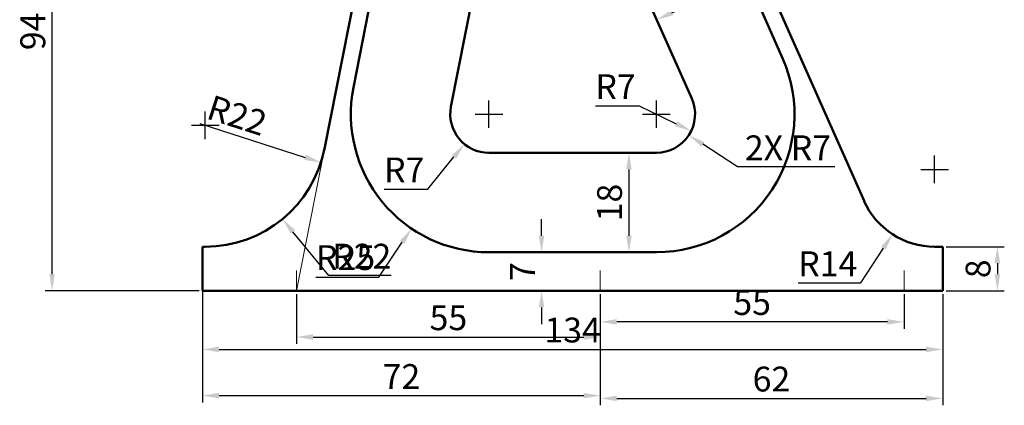
# Model space of a CAD drawing. Units: millimetres. Extents: x 43 to 233, y 2 to 211.
# Tile 1 of 2: x 43 to 221, y 2 to 72. Entities that reach past the tile are written whole.
import ezdxf

# ---------------------------------------------------------------- set-up
doc = ezdxf.new("R2010")
doc.units = ezdxf.units.MM
for name, color, linetype, lineweight in [('M-CONS', 8, 'Continuous', 13), ('M-DIMS', 2, 'Continuous', 25), ('M-OUTL', 7, 'Continuous', 50)]:
    doc.layers.add(name, color=color, linetype=linetype, lineweight=lineweight)
doc.styles.get("Standard").update_dxf_attribs({"font": 'arial.ttf'})
doc.dimstyles.new('ISO-25', dxfattribs={"dimtxt": 4.5, "dimasz": 3, "dimexe": 1.25, "dimexo": 0.625, "dimtad": 1, "dimtoh": 1, "dimdec": 0, "dimtxsty": 'Standard', "dimcen": 2.5, "dimadec": 0, "dimazin": 0, "dimtfac": 1, "dimtdec": 0, "dimtofl": 0, "dimtmove": 0, "dimatfit": 3, "dimfxl": 1, "dimarcsym": 0})

# ---------------------------------------------------------------- blocks, each defined once
blk = doc.blocks.new('*D1')
at = {"layer": 'Defpoints', "color": 0, "transparency": 16777216}
for p in [(75.97, 24.51), (147.97, 23.16), (147.97, 4.19)]:
    blk.add_point(p, dxfattribs=at)
at = {"layer": 'M-DIMS', "color": 0, "lineweight": -2, "transparency": 16777216}
for p, q in [((75.97, 23.88), (75.97, 2.94)), ((147.97, 22.54), (147.97, 2.94)), ((78.97, 4.19), (144.97, 4.19))]:
    blk.add_line(p, q, dxfattribs=at)
at = {"layer": 'M-DIMS', "color": 0, "transparency": 16777216}
for points in [[(78.97, 4.69), (78.97, 3.69), (75.97, 4.19)], [(144.97, 4.69), (144.97, 3.69), (147.97, 4.19)]]:
    blk.add_solid(points, dxfattribs=at)
at = {"layer": 'M-DIMS', "color": 0, "transparency": 16777216, "insert": (111.97, 7.07), "char_height": 4.5, "attachment_point": 5}
blk.add_mtext('72', dxfattribs=at)
blk = doc.blocks.new('*D2')
at = {"layer": 'Defpoints', "color": 0, "transparency": 16777216}
for p in [(147.97, 23.16), (209.97, 23.16), (209.97, 3.69)]:
    blk.add_point(p, dxfattribs=at)
at = {"layer": 'M-DIMS', "color": 0, "lineweight": -2, "transparency": 16777216}
for p, q in [((147.97, 22.54), (147.97, 2.44)), ((209.97, 22.54), (209.97, 2.44)), ((150.97, 3.69), (206.97, 3.69))]:
    blk.add_line(p, q, dxfattribs=at)
at = {"layer": 'M-DIMS', "color": 0, "transparency": 16777216}
for points in [[(150.97, 4.19), (150.97, 3.19), (147.97, 3.69)], [(206.97, 4.19), (206.97, 3.19), (209.97, 3.69)]]:
    blk.add_solid(points, dxfattribs=at)
at = {"layer": 'M-DIMS', "color": 0, "transparency": 16777216, "insert": (178.97, 6.61), "char_height": 4.5, "attachment_point": 5}
blk.add_mtext('62', dxfattribs=at)
blk = doc.blocks.new('*D3')
at = {"layer": 'Defpoints', "color": 0, "transparency": 16777216}
for p in [(137.35, 30.16), (137.35, 23.16), (137.35, 23.16)]:
    blk.add_point(p, dxfattribs=at)
at = {"layer": 'M-DIMS', "color": 0, "lineweight": -2, "transparency": 16777216}
for p, q in [((137.35, 33.16), (137.35, 36.16)), ((137.97, 30.16), (138.6, 30.16)), ((137.97, 23.16), (138.6, 23.16)), ((137.35, 20.16), (137.35, 17.16))]:
    blk.add_line(p, q, dxfattribs=at)
at = {"layer": 'M-DIMS', "color": 0, "transparency": 16777216}
for points in [[(136.85, 33.16), (137.85, 33.16), (137.35, 30.16)], [(136.85, 20.16), (137.85, 20.16), (137.35, 23.16)]]:
    blk.add_solid(points, dxfattribs=at)
at = {"layer": 'M-DIMS', "color": 0, "transparency": 16777216, "insert": (134.47, 26.66), "char_height": 4.5, "attachment_point": 5, "rotation": 90}
blk.add_mtext('7', dxfattribs=at)
blk = doc.blocks.new('*D4')
at = {"layer": 'Defpoints', "color": 0, "transparency": 16777216}
for p in [(209.97, 31.16), (209.97, 23.16), (219.88, 23.16)]:
    blk.add_point(p, dxfattribs=at)
at = {"layer": 'M-DIMS', "color": 0, "lineweight": -2, "transparency": 16777216}
for p, q in [((210.59, 31.16), (221.13, 31.16)), ((219.88, 28.16), (219.88, 26.16)), ((210.59, 23.16), (221.13, 23.16))]:
    blk.add_line(p, q, dxfattribs=at)
at = {"layer": 'M-DIMS', "color": 0, "transparency": 16777216}
for points in [[(219.38, 28.16), (220.38, 28.16), (219.88, 31.16)], [(219.38, 26.16), (220.38, 26.16), (219.88, 23.16)]]:
    blk.add_solid(points, dxfattribs=at)
at = {"layer": 'M-DIMS', "color": 0, "transparency": 16777216, "insert": (216.96, 27.16), "char_height": 4.5, "attachment_point": 5, "rotation": 90}
blk.add_mtext('8', dxfattribs=at)
blk = doc.blocks.new('*D7')
at = {"layer": 'Defpoints', "color": 0, "transparency": 16777216}
for p in [(48.73, 117.16), (87.97, 117.16), (75.97, 23.16)]:
    blk.add_point(p, dxfattribs=at)
at = {"layer": 'M-DIMS', "color": 0, "lineweight": -2, "transparency": 16777216}
for p, q in [((87.34, 117.16), (47.48, 117.16)), ((48.73, 26.16), (48.73, 114.16)), ((75.34, 23.16), (47.48, 23.16))]:
    blk.add_line(p, q, dxfattribs=at)
at = {"layer": 'M-DIMS', "color": 0, "transparency": 16777216}
for points in [[(48.23, 114.16), (49.23, 114.16), (48.73, 117.16)], [(48.23, 26.16), (49.23, 26.16), (48.73, 23.16)]]:
    blk.add_solid(points, dxfattribs=at)
at = {"layer": 'M-DIMS', "color": 0, "transparency": 16777216, "insert": (45.81, 70.16), "char_height": 4.5, "attachment_point": 5, "rotation": 90}
blk.add_mtext('94', dxfattribs=at)
blk = doc.blocks.new('*D9')
at = {"layer": 'Defpoints', "color": 0, "transparency": 16777216}
for p in [(147.97, 23.16), (202.97, 23.16), (147.97, 17.55)]:
    blk.add_point(p, dxfattribs=at)
at = {"layer": 'M-DIMS', "color": 0, "lineweight": -2, "transparency": 16777216}
for p, q in [((147.97, 22.54), (147.97, 16.3)), ((202.97, 22.54), (202.97, 16.3)), ((199.97, 17.55), (150.97, 17.55))]:
    blk.add_line(p, q, dxfattribs=at)
at = {"layer": 'M-DIMS', "color": 0, "transparency": 16777216}
for points in [[(150.97, 18.05), (150.97, 17.05), (147.97, 17.55)], [(199.97, 18.05), (199.97, 17.05), (202.97, 17.55)]]:
    blk.add_solid(points, dxfattribs=at)
at = {"layer": 'M-DIMS', "color": 0, "transparency": 16777216, "insert": (175.47, 20.47), "char_height": 4.5, "attachment_point": 5}
blk.add_mtext('55', dxfattribs=at)
blk = doc.blocks.new('*D10')
at = {"layer": 'Defpoints', "color": 0, "transparency": 16777216}
for p in [(92.97, 23.16), (147.97, 23.16), (147.97, 14.8)]:
    blk.add_point(p, dxfattribs=at)
at = {"layer": 'M-DIMS', "color": 0, "lineweight": -2, "transparency": 16777216}
for p, q in [((92.97, 22.54), (92.97, 13.55)), ((147.97, 22.54), (147.97, 13.55)), ((95.97, 14.8), (144.97, 14.8))]:
    blk.add_line(p, q, dxfattribs=at)
at = {"layer": 'M-DIMS', "color": 0, "transparency": 16777216}
for points in [[(95.97, 15.3), (95.97, 14.3), (92.97, 14.8)], [(144.97, 15.3), (144.97, 14.3), (147.97, 14.8)]]:
    blk.add_solid(points, dxfattribs=at)
at = {"layer": 'M-DIMS', "color": 0, "transparency": 16777216, "insert": (120.47, 17.72), "char_height": 4.5, "attachment_point": 5}
blk.add_mtext('55', dxfattribs=at)
blk = doc.blocks.new('*D16')
at = {"layer": 'Defpoints', "color": 0, "transparency": 16777216}
for p in [(76.45, 53.16), (97.39, 46.42)]:
    blk.add_point(p, dxfattribs=at)
at = {"layer": 'M-DIMS', "color": 0, "lineweight": -2, "transparency": 16777216}
blk.add_line((75.46, 53.48), (94.54, 47.34), dxfattribs=at)
at = {"layer": 'M-DIMS', "color": 0, "transparency": 16777216}
blk.add_solid([(94.69, 47.82), (94.39, 46.87), (97.39, 46.42)], dxfattribs=at)
at = {"layer": 'M-DIMS', "color": 0, "transparency": 16777216, "insert": (82.04, 54.39), "char_height": 4.5, "attachment_point": 5, "rotation": 342.1638}
blk.add_mtext('R22', dxfattribs=at)
blk = doc.blocks.new('*D21')
at = {"layer": 'Defpoints', "color": 0, "transparency": 16777216}
for p in [(127.81, 55.16), (113.81, 34.45)]:
    blk.add_point(p, dxfattribs=at)
at = {"layer": 'M-DIMS', "color": 0, "lineweight": -2, "transparency": 16777216}
for p, q in [((127.81, 52.66), (127.81, 57.66)), ((125.31, 55.16), (130.31, 55.16)), ((107.87, 25.67), (112.13, 31.97)), ((96.46, 25.67), (107.87, 25.67))]:
    blk.add_line(p, q, dxfattribs=at)
at = {"layer": 'M-DIMS', "color": 0, "transparency": 16777216}
blk.add_solid([(111.71, 32.25), (112.54, 31.69), (113.81, 34.45)], dxfattribs=at)
at = {"layer": 'M-DIMS', "color": 0, "transparency": 16777216, "insert": (101.85, 28.6), "char_height": 4.5, "attachment_point": 5}
blk.add_mtext('R25', dxfattribs=at)
blk = doc.blocks.new('*D22')
at = {"layer": 'Defpoints', "color": 0, "transparency": 16777216}
for p in [(127.81, 55.16), (123.38, 49.74)]:
    blk.add_point(p, dxfattribs=at)
at = {"layer": 'M-DIMS', "color": 0, "lineweight": -2, "transparency": 16777216}
for p, q in [((127.81, 52.66), (127.81, 57.66)), ((125.31, 55.16), (130.31, 55.16)), ((116.73, 41.61), (121.48, 47.42)), ((108.85, 41.61), (116.73, 41.61))]:
    blk.add_line(p, q, dxfattribs=at)
at = {"layer": 'M-DIMS', "color": 0, "transparency": 16777216}
blk.add_solid([(121.09, 47.73), (121.87, 47.1), (123.38, 49.74)], dxfattribs=at)
at = {"layer": 'M-DIMS', "color": 0, "transparency": 16777216, "insert": (112.48, 44.48), "char_height": 4.5, "attachment_point": 5}
blk.add_mtext('R7', dxfattribs=at)
blk = doc.blocks.new('*D23')
at = {"layer": 'Defpoints', "color": 0, "transparency": 16777216}
for p in [(158.14, 55.16), (164.45, 52.12)]:
    blk.add_point(p, dxfattribs=at)
at = {"layer": 'M-DIMS', "color": 0, "lineweight": -2, "transparency": 16777216}
for p, q in [((147.11, 56.68), (154.99, 56.68)), ((154.99, 56.68), (161.74, 53.42))]:
    blk.add_line(p, q, dxfattribs=at)
at = {"layer": 'M-DIMS', "color": 0, "transparency": 16777216}
blk.add_solid([(161.96, 53.87), (161.53, 52.97), (164.45, 52.12)], dxfattribs=at)
at = {"layer": 'M-DIMS', "color": 0, "transparency": 16777216, "insert": (150.74, 59.56), "char_height": 4.5, "attachment_point": 5}
blk.add_mtext('R7', dxfattribs=at)
blk = doc.blocks.new('*D24')
at = {"layer": 'Defpoints', "color": 0, "transparency": 16777216}
for p in [(174.65, 79.59), (179.84, 67.89), (163.39, 60.6)]:
    blk.add_point(p, dxfattribs=at)
at = {"layer": 'M-DIMS', "color": 0, "lineweight": -2, "transparency": 16777216}
for p, q in [((179.59, 68.46), (174.15, 80.74)), ((160.94, 73.51), (171.91, 78.38)), ((163.14, 61.17), (157.69, 73.44))]:
    blk.add_line(p, q, dxfattribs=at)
at = {"layer": 'M-DIMS', "color": 0, "transparency": 16777216}
for points in [[(171.71, 78.83), (172.11, 77.92), (174.65, 79.59)], [(160.74, 73.97), (161.15, 73.05), (158.2, 72.29)]]:
    blk.add_solid(points, dxfattribs=at)
at = {"layer": 'M-DIMS', "color": 0, "transparency": 16777216, "insert": (165.24, 78.62), "char_height": 4.5, "attachment_point": 5, "rotation": 23.9196}
blk.add_mtext('18', dxfattribs=at)
blk = doc.blocks.new('*D30')
at = {"layer": 'Defpoints', "color": 0, "transparency": 16777216}
for p in [(153.44, 48.16), (153.16, 30.16), (153.44, 30.16)]:
    blk.add_point(p, dxfattribs=at)
at = {"layer": 'M-DIMS', "color": 0, "lineweight": -2, "transparency": 16777216}
for p, q in [((152.82, 48.16), (151.91, 48.16)), ((153.16, 45.16), (153.16, 33.16)), ((152.82, 30.16), (151.91, 30.16))]:
    blk.add_line(p, q, dxfattribs=at)
at = {"layer": 'M-DIMS', "color": 0, "transparency": 16777216}
for points in [[(152.66, 45.16), (153.66, 45.16), (153.16, 48.16)], [(152.66, 33.16), (153.66, 33.16), (153.16, 30.16)]]:
    blk.add_solid(points, dxfattribs=at)
at = {"layer": 'M-DIMS', "color": 0, "transparency": 16777216, "insert": (150.24, 39.16), "char_height": 4.5, "attachment_point": 5, "rotation": 90}
blk.add_mtext('18', dxfattribs=at)
blk = doc.blocks.new('*D31')
at = {"layer": 'Defpoints', "color": 0, "transparency": 16777216}
for p in [(75.97, 23.16), (209.97, 23.16), (209.97, 12.56)]:
    blk.add_point(p, dxfattribs=at)
at = {"layer": 'M-DIMS', "color": 0, "lineweight": -2, "transparency": 16777216}
for p, q in [((75.97, 22.54), (75.97, 11.31)), ((209.97, 22.54), (209.97, 11.31)), ((78.97, 12.56), (206.97, 12.56))]:
    blk.add_line(p, q, dxfattribs=at)
at = {"layer": 'M-DIMS', "color": 0, "transparency": 16777216}
for points in [[(78.97, 13.06), (78.97, 12.06), (75.97, 12.56)], [(206.97, 13.06), (206.97, 12.06), (209.97, 12.56)]]:
    blk.add_solid(points, dxfattribs=at)
at = {"layer": 'M-DIMS', "color": 0, "transparency": 16777216, "insert": (142.97, 15.49), "char_height": 4.5, "attachment_point": 5}
blk.add_mtext('134', dxfattribs=at)
blk = doc.blocks.new('*D41')
at = {"layer": 'Defpoints', "color": 0, "transparency": 16777216}
for p in [(158.14, 55.16), (164.01, 51.35)]:
    blk.add_point(p, dxfattribs=at)
at = {"layer": 'M-DIMS', "color": 0, "lineweight": -2, "transparency": 16777216}
for p, q in [((158.14, 52.66), (158.14, 57.66)), ((155.64, 55.16), (160.64, 55.16)), ((172.83, 45.61), (166.52, 49.71)), ((190.46, 45.61), (172.83, 45.61))]:
    blk.add_line(p, q, dxfattribs=at)
at = {"layer": 'M-DIMS', "color": 0, "transparency": 16777216}
blk.add_solid([(166.8, 50.13), (166.25, 49.29), (164.01, 51.35)], dxfattribs=at)
at = {"layer": 'M-DIMS', "color": 0, "transparency": 16777216, "insert": (181.96, 48.49), "char_height": 4.5, "attachment_point": 5}
blk.add_mtext('2X R7', dxfattribs=at)
blk = doc.blocks.new('*D42')
at = {"layer": 'Defpoints', "color": 0, "transparency": 16777216}
for p in [(76.45, 53.16), (90.43, 36.17)]:
    blk.add_point(p, dxfattribs=at)
at = {"layer": 'M-DIMS', "color": 0, "lineweight": -2, "transparency": 16777216}
for p, q in [((76.45, 50.66), (76.45, 55.66)), ((73.95, 53.16), (78.95, 53.16)), ((98.81, 25.97), (92.33, 33.85)), ((110.14, 25.97), (98.81, 25.97))]:
    blk.add_line(p, q, dxfattribs=at)
at = {"layer": 'M-DIMS', "color": 0, "transparency": 16777216}
blk.add_solid([(92.72, 34.17), (91.94, 33.53), (90.43, 36.17)], dxfattribs=at)
at = {"layer": 'M-DIMS', "color": 0, "transparency": 16777216, "insert": (104.79, 28.86), "char_height": 4.5, "attachment_point": 5}
blk.add_mtext('R22', dxfattribs=at)
blk = doc.blocks.new('*D43')
at = {"layer": 'Defpoints', "color": 0, "transparency": 16777216}
for p in [(208.52, 45.16), (200.89, 33.43)]:
    blk.add_point(p, dxfattribs=at)
at = {"layer": 'M-DIMS', "color": 0, "lineweight": -2, "transparency": 16777216}
for p, q in [((208.52, 42.66), (208.52, 47.66)), ((206.02, 45.16), (211.02, 45.16)), ((195.15, 24.61), (199.25, 30.91)), ((183.8, 24.61), (195.15, 24.61))]:
    blk.add_line(p, q, dxfattribs=at)
at = {"layer": 'M-DIMS', "color": 0, "transparency": 16777216}
blk.add_solid([(198.84, 31.18), (199.67, 30.64), (200.89, 33.43)], dxfattribs=at)
at = {"layer": 'M-DIMS', "color": 0, "transparency": 16777216, "insert": (189.16, 27.49), "char_height": 4.5, "attachment_point": 5}
blk.add_mtext('R14', dxfattribs=at)

msp = doc.modelspace()

# ---------------------------------------------------------------- linework, layer by layer
at = {"layer": 'M-CONS'}
for p, q in [((92.97, 23.16), (98.04, 48.91)), ((92.97, 23.16), (92.97, 26.86)), ((147.97, 23.16), (147.97, 26.86)), ((202.97, 23.16), (202.97, 26.86))]:
    msp.add_line(p, q, dxfattribs=at)
at = {"layer": 'M-OUTL'}
for p, q in [((164.54, 58), (147.38, 96.68)), ((120.94, 56.51), (128.43, 94.56)), ((195.73, 39.49), (173.28, 90.08)), ((180.99, 65.3), (170.54, 88.87)), ((98.04, 48.91), (103.65, 77.39)), ((103.28, 59.99), (106.59, 76.81)), ((158.14, 48.16), (127.81, 48.16)), ((75.97, 23.16), (75.97, 31.16)), ((75.97, 31.16), (76.45, 31.16)), ((209.97, 31.16), (208.52, 31.16)), ((209.97, 23.16), (209.97, 31.16)), ((158.14, 30.16), (127.81, 30.16)), ((209.97, 23.16), (75.97, 23.16))]:
    msp.add_line(p, q, dxfattribs=at)
for centre, radius, start, end in [((158.14, 55.16), 25, 270, 23.9196), ((127.81, 55.16), 25, 168.8574, 270), ((158.14, 55.16), 7, 270, 23.9196), ((127.81, 55.16), 7, 168.8574, 270), ((76.45, 53.16), 22, 270, 348.8574), ((208.52, 45.16), 14, 203.9196, 270)]:
    msp.add_arc(centre, radius, start, end, dxfattribs=at)

# ---------------------------------------------------------------- dimensions: what is measured, and where the dimension line sits
at = {"layer": 'M-DIMS'}
for base, p1, p2, picture, middle in [((48.73, 117.16), (75.97, 23.16), (87.97, 117.16), '*D7', (45.81, 70.16)), ((153.16, 30.16), (153.44, 48.16), (153.44, 30.16), '*D30', (150.24, 39.16)), ((137.35, 23.16), (137.35, 30.16), (137.35, 23.16), '*D3', (134.47, 26.66)), ((219.88, 23.16), (209.97, 31.16), (209.97, 23.16), '*D4', (216.96, 27.16))]:
    dim = msp.add_linear_dim(base=base, p1=p1, p2=p2, angle=90, dimstyle='ISO-25', override={"dimclrd": 0, "dimclre": 0, "dimclrt": 0}, dxfattribs=at)
    dim.commit()
    dim.dimension.update_dxf_attribs({"geometry": picture, "text_midpoint": middle})
dim = msp.add_aligned_dim(p1=(163.39, 60.6), p2=(179.84, 67.89), distance=12.8, dimstyle='ISO-25', override={"dimclrd": 0, "dimclre": 0, "dimclrt": 0}, dxfattribs=at)
dim.commit()
dim.dimension.update_dxf_attribs({"geometry": '*D24', "text_midpoint": (165.24, 78.62)})
for center, mpoint, override, picture, middle in [((158.14, 55.16), (164.45, 52.12), {"dimclrd": 0, "dimclre": 0, "dimclrt": 0}, '*D23', (150.74, 56.68)), ((76.45, 53.16), (97.39, 46.42), {"dimclrd": 0, "dimclre": 0, "dimclrt": 0}, '*D16', (81.15, 51.65)), ((76.45, 53.16), (90.43, 36.17), {"dimdec": 0, "dimlfac": 1, "dimrnd": 0, "dimzin": 0, "dimdsep": 46, "dimlunit": 2}, '*D42', (104.79, 25.97))]:
    dim = msp.add_radius_dim(center=center, mpoint=mpoint, dimstyle='ISO-25', override=override, dxfattribs=at)
    dim.commit()
    dim.dimension.update_dxf_attribs({"geometry": picture, "text_midpoint": middle, "dimtype": 164})
for center, mpoint, override, picture, middle in [((127.81, 55.16), (113.81, 34.45), {"dimclrd": 0, "dimclre": 0, "dimclrt": 0}, '*D21', (101.85, 28.6)), ((127.81, 55.16), (123.38, 49.74), {"dimclrd": 0, "dimclre": 0, "dimclrt": 0}, '*D22', (112.48, 44.48)), ((208.52, 45.16), (200.89, 33.43), {"dimdec": 0, "dimlfac": 1, "dimrnd": 0, "dimzin": 0, "dimdsep": 46, "dimlunit": 2}, '*D43', (189.16, 27.49))]:
    dim = msp.add_radius_dim(center=center, mpoint=mpoint, dimstyle='ISO-25', override=override, dxfattribs=at)
    dim.commit()
    dim.dimension.update_dxf_attribs({"geometry": picture, "text_midpoint": middle})
dim = msp.add_radius_dim(center=(158.14, 55.16), mpoint=(164.01, 51.35), text='2X <>', dimstyle='ISO-25', override={"dimdec": 0, "dimlfac": 1, "dimrnd": 0, "dimzin": 0, "dimdsep": 46, "dimlunit": 2}, dxfattribs=at)
dim.commit()
dim.dimension.update_dxf_attribs({"geometry": '*D41', "text_midpoint": (181.96, 48.49)})
for base, p1, p2, override, picture, middle in [((147.97, 4.19), (75.97, 24.51), (147.97, 23.16), {"dimclrd": 0, "dimclre": 0, "dimclrt": 0}, '*D1', (111.97, 7.07)), ((147.97, 17.55), (202.97, 23.16), (147.97, 23.16), {"dimclrd": 0, "dimclre": 0, "dimclrt": 0}, '*D9', (175.47, 20.47)), ((209.97, 12.56), (75.97, 23.16), (209.97, 23.16), {"dimdec": 0, "dimlfac": 1, "dimrnd": 0, "dimzin": 0, "dimdsep": 46, "dimlunit": 2}, '*D31', (142.97, 15.49)), ((147.97, 14.8), (92.97, 23.16), (147.97, 23.16), {"dimclrd": 0, "dimclre": 0, "dimclrt": 0}, '*D10', (120.47, 17.72)), ((209.97, 3.69), (147.97, 23.16), (209.97, 23.16), {"dimclrd": 0, "dimclre": 0, "dimclrt": 0}, '*D2', (178.97, 6.61))]:
    dim = msp.add_linear_dim(base=base, p1=p1, p2=p2, dimstyle='ISO-25', override=override, dxfattribs=at)
    dim.commit()
    dim.dimension.update_dxf_attribs({"geometry": picture, "text_midpoint": middle})

doc.saveas('drawing.dxf')
